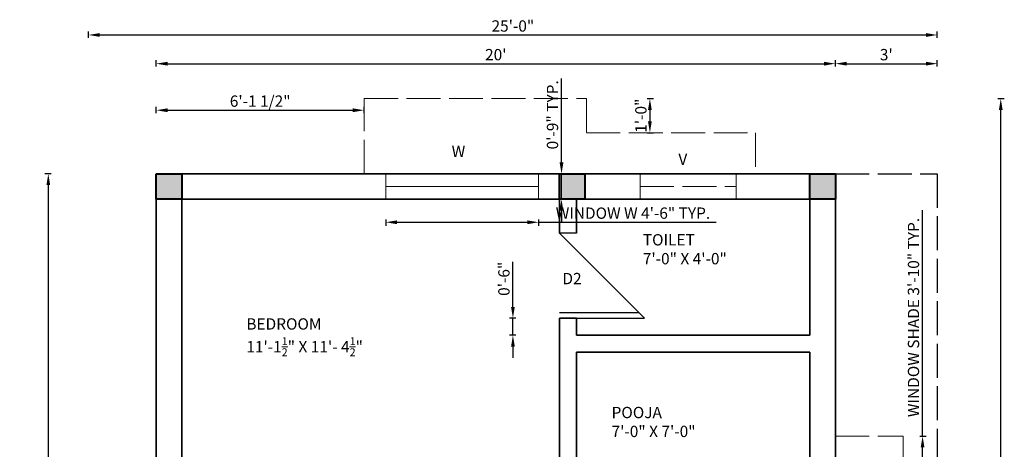
# Model space of a CAD drawing. Units: inches. Extents: x -52 to 299, y -380 to 67.
# Tile 2 of 2: x -49 to 299, y -84 to 67. Entities that reach past the tile are written whole.
import ezdxf

# ---------------------------------------------------------------- set-up
doc = ezdxf.new("R2010")
doc.units = ezdxf.units.IN
doc.linetypes.add('ACAD_ISO02W100', pattern=[15, 12, -3])
for name, color, linetype, lineweight in [('A-ANNO-DIMS', 2, 'Continuous', 18), ('A-ANNO-TEXT', 7, 'Continuous', 18), ('A-AREA-IDEN', 7, 'Continuous', 18), ('A-COLS', 7, 'Continuous', 40), ('A-DOOR', 3, 'Continuous', 25), ('A-GLAZ', 4, 'Continuous', 18), ('A-GLAZ-VENT', 4, 'ACAD_ISO02W100', 18), ('A-ROOF-OVHD', 8, 'ACAD_ISO02W100', 18), ('A-WALL', 7, 'Continuous', 35), ('C-PROP', 8, 'ACAD_ISO02W100', 25)]:
    doc.layers.add(name, color=color, linetype=linetype, lineweight=lineweight)
doc.styles.get("Standard").update_dxf_attribs({"font": 'arial.ttf'})
doc.dimstyles.new('ISO-25', dxfattribs={"dimtxt": 4, "dimasz": 4, "dimexe": 1.25, "dimexo": 0.625, "dimtad": 1, "dimlunit": 4, "dimtxsty": 'Standard', "dimcen": 2.5, "dimadec": 0, "dimazin": 0, "dimtfac": 1, "dimtmove": 0, "dimatfit": 3, "dimfxl": 1, "dimfxlon": 1, "dimarcsym": 0})

# ---------------------------------------------------------------- blocks, each defined once
blk = doc.blocks.new('*D1')
at = {"layer": 'A-ANNO-DIMS', "color": 0, "lineweight": -2, "transparency": 16777216}
for p, q in [((-0.38, 50.68), (-0.38, 52.93)), ((239.62, 50.68), (239.62, 52.93)), ((3.62, 51.68), (235.62, 51.68))]:
    blk.add_line(p, q, dxfattribs=at)
at = {"layer": 'A-ANNO-DIMS', "color": 0, "transparency": 16777216}
for points in [[(3.62, 52.35), (3.62, 51.01), (-0.38, 51.68)], [(235.62, 52.35), (235.62, 51.01), (239.62, 51.68)]]:
    blk.add_solid(points, dxfattribs=at)
at = {"layer": 'Defpoints', "color": 0, "transparency": 16777216}
for p in [(239.62, 51.68), (-0.38, 12.8), (239.62, 12.8)]:
    blk.add_point(p, dxfattribs=at)
at = {"layer": 'A-ANNO-DIMS', "color": 0, "transparency": 16777216, "insert": (119.62, 54.35), "char_height": 4, "attachment_point": 5}
blk.add_mtext("20'", dxfattribs=at)
blk = doc.blocks.new('*D2')
at = {"layer": 'A-ANNO-DIMS', "color": 0, "lineweight": -2, "transparency": 16777216}
for p, q in [((239.62, 50.68), (239.62, 52.93)), ((275.62, 50.68), (275.62, 52.93)), ((243.62, 51.68), (271.62, 51.68))]:
    blk.add_line(p, q, dxfattribs=at)
at = {"layer": 'A-ANNO-DIMS', "color": 0, "transparency": 16777216}
for points in [[(243.62, 52.35), (243.62, 51.01), (239.62, 51.68)], [(271.62, 52.35), (271.62, 51.01), (275.62, 51.68)]]:
    blk.add_solid(points, dxfattribs=at)
at = {"layer": 'Defpoints', "color": 0, "transparency": 16777216}
for p in [(275.62, 51.68), (239.62, 12.8), (275.62, 12.8)]:
    blk.add_point(p, dxfattribs=at)
at = {"layer": 'A-ANNO-DIMS', "color": 0, "transparency": 16777216, "insert": (257.62, 54.35), "char_height": 4, "attachment_point": 5}
blk.add_mtext("3'", dxfattribs=at)
blk = doc.blocks.new('*D3')
at = {"layer": 'A-ANNO-DIMS', "color": 0, "lineweight": -2, "transparency": 16777216}
for p, q in [((-37.52, 12.8), (-39.77, 12.8)), ((-38.52, 8.8), (-38.52, -278.7)), ((-37.52, -282.7), (-39.77, -282.7))]:
    blk.add_line(p, q, dxfattribs=at)
at = {"layer": 'A-ANNO-DIMS', "color": 0, "transparency": 16777216}
for points in [[(-39.19, 8.8), (-37.85, 8.8), (-38.52, 12.8)], [(-39.19, -278.7), (-37.85, -278.7), (-38.52, -282.7)]]:
    blk.add_solid(points, dxfattribs=at)
at = {"layer": 'Defpoints', "color": 0, "transparency": 16777216}
for p in [(-0.38, 12.8), (-38.52, -282.7), (-0.38, -282.7)]:
    blk.add_point(p, dxfattribs=at)
at = {"layer": 'A-ANNO-DIMS', "color": 0, "transparency": 16777216, "insert": (-43.83, -134.95), "char_height": 4, "attachment_point": 5, "rotation": 90}
blk.add_mtext('24\'-7{\\H1x;\\S1/2;}"', dxfattribs=at)
blk = doc.blocks.new('COL-9X9')
h = blk.add_hatch(color=256)
h.dxf.hatch_style = 1
h.paths.add_polyline_path([(0, 0), (9, 0), (9, 9), (0, 9)])
blk.add_lwpolyline([(0, 9), (9, 9), (9, 0), (0, 0)], close=True)
blk = doc.blocks.new('WIN-54')
blk.add_line((0, 4.5), (54, 4.5))
blk.add_lwpolyline([(0, 9), (54, 9), (54, 0), (0, 0)], close=True)
blk = doc.blocks.new('DOOR-D2-30')
for p, q in [((0, 0), (0, 30)), ((30, 0), (0, 30)), ((2, 0), (2, 28)), ((0, 6), (0, 0)), ((30, 6), (30, 0))]:
    blk.add_line(p, q)
blk = doc.blocks.new('WINDOW-SHADE-34')
blk.add_lwpolyline([(0, 45.87), (23.94, 45.87), (23.94, 0), (0, 0)], close=True)
blk = doc.blocks.new('*D12')
at = {"layer": 'A-ANNO-DIMS', "color": 0, "lineweight": -2, "transparency": 16777216}
for p, q in [((80.75, -3.3), (80.75, -5.55)), ((134.75, -3.3), (134.75, -5.55)), ((84.75, -4.3), (130.75, -4.3)), ((134.75, -4.3), (197.44, -4.3))]:
    blk.add_line(p, q, dxfattribs=at)
at = {"layer": 'A-ANNO-DIMS', "color": 0, "transparency": 16777216}
for points in [[(84.75, -3.63), (84.75, -4.97), (80.75, -4.3)], [(130.75, -3.63), (130.75, -4.97), (134.75, -4.3)]]:
    blk.add_solid(points, dxfattribs=at)
at = {"layer": 'Defpoints', "color": 0, "transparency": 16777216}
for p in [(80.75, 3.8), (134.75, 3.8), (134.75, -4.3)]:
    blk.add_point(p, dxfattribs=at)
at = {"layer": 'A-ANNO-DIMS', "color": 0, "transparency": 16777216, "insert": (168.09, -1.6), "char_height": 4, "attachment_point": 5}
blk.add_mtext('WINDOW W 4\'-6" TYP.', dxfattribs=at)
blk = doc.blocks.new('*D13')
at = {"layer": 'A-ANNO-DIMS', "color": 0, "lineweight": -2, "transparency": 16777216}
for p, q in [((142.85, 16.8), (142.85, 46.43)), ((141.85, 12.8), (144.1, 12.8)), ((142.85, 3.8), (142.85, 12.8)), ((141.85, 3.8), (144.1, 3.8)), ((142.85, -0.2), (142.85, -4.2))]:
    blk.add_line(p, q, dxfattribs=at)
at = {"layer": 'A-ANNO-DIMS', "color": 0, "transparency": 16777216}
for points in [[(142.18, 16.8), (143.51, 16.8), (142.85, 12.8)], [(142.18, -0.2), (143.51, -0.2), (142.85, 3.8)]]:
    blk.add_solid(points, dxfattribs=at)
at = {"layer": 'Defpoints', "color": 0, "transparency": 16777216}
for p in [(134.75, 12.8), (142.85, 12.8), (134.75, 3.8)]:
    blk.add_point(p, dxfattribs=at)
at = {"layer": 'A-ANNO-DIMS', "color": 0, "transparency": 16777216, "insert": (140.18, 33.62), "char_height": 4, "attachment_point": 5, "rotation": 90}
blk.add_mtext('0\'-9" TYP.', dxfattribs=at)
blk = doc.blocks.new('*D18')
at = {"layer": 'A-ANNO-DIMS', "color": 0, "lineweight": -2, "transparency": 16777216}
for p, q in [((270.45, -79.8), (270.45, -0.02)), ((269.45, -79.8), (271.7, -79.8)), ((270.45, -121.66), (270.45, -83.8)), ((269.45, -125.66), (271.7, -125.66))]:
    blk.add_line(p, q, dxfattribs=at)
at = {"layer": 'A-ANNO-DIMS', "color": 0, "transparency": 16777216}
for points in [[(269.78, -83.8), (271.11, -83.8), (270.45, -79.8)], [(269.78, -121.66), (271.11, -121.66), (270.45, -125.66)]]:
    blk.add_solid(points, dxfattribs=at)
at = {"layer": 'Defpoints', "color": 0, "transparency": 16777216}
for p in [(263.57, -79.8), (270.45, -79.8), (263.57, -125.66)]:
    blk.add_point(p, dxfattribs=at)
at = {"layer": 'A-ANNO-DIMS', "color": 0, "transparency": 16777216, "insert": (267.75, -37.91), "char_height": 4, "attachment_point": 5, "rotation": 90}
blk.add_mtext('WINDOW SHADE 3\'-10" TYP.', dxfattribs=at)
blk = doc.blocks.new('*D20')
at = {"layer": 'A-ANNO-DIMS', "color": 0, "lineweight": -2, "transparency": 16777216}
for p, q in [((-24.32, 60.81), (-24.32, 63.06)), ((275.62, 60.81), (275.62, 63.06)), ((-20.32, 61.81), (271.62, 61.81))]:
    blk.add_line(p, q, dxfattribs=at)
at = {"layer": 'A-ANNO-DIMS', "color": 0, "transparency": 16777216}
for points in [[(-20.32, 62.47), (-20.32, 61.14), (-24.32, 61.81)], [(271.62, 62.47), (271.62, 61.14), (275.62, 61.81)]]:
    blk.add_solid(points, dxfattribs=at)
at = {"layer": 'Defpoints', "color": 0, "transparency": 16777216}
for p in [(275.62, 61.81), (275.62, 12.8), (-24.32, -215.36)]:
    blk.add_point(p, dxfattribs=at)
at = {"layer": 'A-ANNO-DIMS', "color": 0, "transparency": 16777216, "insert": (125.65, 64.47), "char_height": 4, "attachment_point": 5}
blk.add_mtext('25\'-0"', dxfattribs=at)
blk = doc.blocks.new('*D21')
at = {"layer": 'A-ANNO-DIMS', "color": 0, "lineweight": -2, "transparency": 16777216}
for p, q in [((297.07, 39.36), (299.32, 39.36)), ((298.07, -350.7), (298.07, 35.36)), ((297.07, -354.7), (299.32, -354.7))]:
    blk.add_line(p, q, dxfattribs=at)
at = {"layer": 'A-ANNO-DIMS', "color": 0, "transparency": 16777216}
for points in [[(297.41, 35.36), (298.74, 35.36), (298.07, 39.36)], [(297.41, -350.7), (298.74, -350.7), (298.07, -354.7)]]:
    blk.add_solid(points, dxfattribs=at)
at = {"layer": 'Defpoints', "color": 0, "transparency": 16777216}
for p in [(151.63, 39.36), (298.07, 39.36), (275.62, -354.7)]:
    blk.add_point(p, dxfattribs=at)
at = {"layer": 'A-ANNO-DIMS', "color": 0, "transparency": 16777216, "insert": (295.4, -157.67), "char_height": 4, "attachment_point": 5, "rotation": 90}
blk.add_mtext('32\'-10"', dxfattribs=at)
blk = doc.blocks.new('*D24')
at = {"layer": 'A-ANNO-DIMS', "color": 0, "lineweight": -2, "transparency": 16777216}
for p, q in [((8.62, -376.15), (8.62, -378.4)), ((12.62, -377.15), (76.75, -377.15)), ((80.75, -376.15), (80.75, -378.4))]:
    blk.add_line(p, q, dxfattribs=at)
at = {"layer": 'A-ANNO-DIMS', "color": 0, "transparency": 16777216}
for points in [[(12.62, -376.48), (12.62, -377.82), (8.62, -377.15)], [(76.75, -376.48), (76.75, -377.82), (80.75, -377.15)]]:
    blk.add_solid(points, dxfattribs=at)
at = {"layer": 'Defpoints', "color": 0, "transparency": 16777216}
for p in [(8.62, 3.8), (80.75, 3.8), (80.75, -377.15)]:
    blk.add_point(p, dxfattribs=at)
at = {"layer": 'A-ANNO-DIMS', "color": 0, "transparency": 16777216, "insert": (44.69, -374.48), "char_height": 4, "attachment_point": 5}
blk.add_mtext('6\'-0"', dxfattribs=at)
blk = doc.blocks.new('*D25')
at = {"layer": 'A-ANNO-DIMS', "color": 0, "lineweight": -2, "transparency": 16777216}
for p, q in [((170.58, -376.15), (170.58, -378.4)), ((174.58, -377.15), (200.58, -377.15)), ((204.58, -376.15), (204.58, -378.4))]:
    blk.add_line(p, q, dxfattribs=at)
at = {"layer": 'A-ANNO-DIMS', "color": 0, "transparency": 16777216}
for points in [[(174.58, -376.48), (174.58, -377.82), (170.58, -377.15)], [(200.58, -376.48), (200.58, -377.82), (204.58, -377.15)]]:
    blk.add_solid(points, dxfattribs=at)
at = {"layer": 'Defpoints', "color": 0, "transparency": 16777216}
for p in [(170.58, 3.8), (204.58, 3.8), (204.58, -377.15)]:
    blk.add_point(p, dxfattribs=at)
at = {"layer": 'A-ANNO-DIMS', "color": 0, "transparency": 16777216, "insert": (187.58, -374.48), "char_height": 4, "attachment_point": 5}
blk.add_mtext('2\'-10"', dxfattribs=at)
blk = doc.blocks.new('*D26')
at = {"layer": 'A-ANNO-DIMS', "color": 0, "lineweight": -2, "transparency": 16777216}
for p, q in [((204.58, -376.15), (204.58, -378.4)), ((208.58, -377.15), (226.62, -377.15)), ((230.62, -376.15), (230.62, -378.4))]:
    blk.add_line(p, q, dxfattribs=at)
at = {"layer": 'A-ANNO-DIMS', "color": 0, "transparency": 16777216}
for points in [[(208.58, -376.48), (208.58, -377.82), (204.58, -377.15)], [(226.62, -376.48), (226.62, -377.82), (230.62, -377.15)]]:
    blk.add_solid(points, dxfattribs=at)
at = {"layer": 'Defpoints', "color": 0, "transparency": 16777216}
for p in [(204.58, 3.8), (230.62, 3.8), (230.62, -377.15)]:
    blk.add_point(p, dxfattribs=at)
at = {"layer": 'A-ANNO-DIMS', "color": 0, "transparency": 16777216, "insert": (217.6, -374.52), "char_height": 4, "attachment_point": 5}
blk.add_mtext('2\'-2"', dxfattribs=at)
blk = doc.blocks.new('*D36')
at = {"layer": 'A-ANNO-DIMS', "color": 0, "lineweight": -2, "transparency": 16777216}
for p, q in [((125.67, -34.2), (125.67, -18.32)), ((126.67, -38.2), (124.42, -38.2)), ((125.67, -44.2), (125.67, -38.2)), ((126.67, -44.2), (124.42, -44.2)), ((125.67, -48.2), (125.67, -52.2))]:
    blk.add_line(p, q, dxfattribs=at)
at = {"layer": 'A-ANNO-DIMS', "color": 0, "transparency": 16777216}
for points in [[(125.01, -34.2), (126.34, -34.2), (125.67, -38.2)], [(125.01, -48.2), (126.34, -48.2), (125.67, -44.2)]]:
    blk.add_solid(points, dxfattribs=at)
at = {"layer": 'Defpoints', "color": 0, "transparency": 16777216}
for p in [(125.67, -38.2), (148.12, -38.2), (148.12, -44.2)]:
    blk.add_point(p, dxfattribs=at)
at = {"layer": 'A-ANNO-DIMS', "color": 0, "transparency": 16777216, "insert": (123.01, -24.26), "char_height": 4, "attachment_point": 5, "rotation": 90}
blk.add_mtext('0\'-6"', dxfattribs=at)
blk = doc.blocks.new('*D40')
at = {"layer": 'A-ANNO-DIMS', "color": 0, "lineweight": -2, "transparency": 16777216}
for p, q in [((173.08, 39.36), (175.33, 39.36)), ((174.08, 35.36), (174.08, 31.28)), ((173.08, 27.28), (175.33, 27.28))]:
    blk.add_line(p, q, dxfattribs=at)
at = {"layer": 'A-ANNO-DIMS', "color": 0, "transparency": 16777216}
for points in [[(173.41, 35.36), (174.74, 35.36), (174.08, 39.36)], [(173.41, 31.28), (174.74, 31.28), (174.08, 27.28)]]:
    blk.add_solid(points, dxfattribs=at)
at = {"layer": 'Defpoints', "color": 0, "transparency": 16777216}
for p in [(151.63, 39.36), (151.63, 27.28), (174.08, 27.28)]:
    blk.add_point(p, dxfattribs=at)
at = {"layer": 'A-ANNO-DIMS', "color": 0, "transparency": 16777216, "insert": (171.41, 33.32), "char_height": 4, "attachment_point": 5, "rotation": 90}
blk.add_mtext('1\'-0"', dxfattribs=at)
blk = doc.blocks.new('*D41')
at = {"layer": 'A-ANNO-DIMS', "color": 0, "lineweight": -2, "transparency": 16777216}
for p, q in [((-0.38, 34.25), (-0.38, 36.5)), ((3.62, 35.25), (69.09, 35.25)), ((73.09, 34.25), (73.09, 36.5))]:
    blk.add_line(p, q, dxfattribs=at)
at = {"layer": 'A-ANNO-DIMS', "color": 0, "transparency": 16777216}
for points in [[(3.62, 35.92), (3.62, 34.58), (-0.38, 35.25)], [(69.09, 35.92), (69.09, 34.58), (73.09, 35.25)]]:
    blk.add_solid(points, dxfattribs=at)
at = {"layer": 'Defpoints', "color": 0, "transparency": 16777216}
for p in [(73.09, 35.25), (-0.38, 12.8), (73.09, 12.8)]:
    blk.add_point(p, dxfattribs=at)
at = {"layer": 'A-ANNO-DIMS', "color": 0, "transparency": 16777216, "insert": (36.36, 37.94), "char_height": 4, "attachment_point": 5}
blk.add_mtext('6\'-1 1/2"', dxfattribs=at)
blk = doc.blocks.new('*D42')
at = {"layer": 'A-ANNO-DIMS', "color": 0, "lineweight": -2, "transparency": 16777216}
for p, q in [((73.09, -376.15), (73.09, -378.4)), ((77.09, -377.15), (147.63, -377.15)), ((151.63, -376.15), (151.63, -378.4))]:
    blk.add_line(p, q, dxfattribs=at)
at = {"layer": 'A-ANNO-DIMS', "color": 0, "transparency": 16777216}
for points in [[(77.09, -376.48), (77.09, -377.82), (73.09, -377.15)], [(147.63, -376.48), (147.63, -377.82), (151.63, -377.15)]]:
    blk.add_solid(points, dxfattribs=at)
at = {"layer": 'Defpoints', "color": 0, "transparency": 16777216}
for p in [(73.09, 39.36), (151.63, 39.36), (151.63, -377.15)]:
    blk.add_point(p, dxfattribs=at)
at = {"layer": 'A-ANNO-DIMS', "color": 0, "transparency": 16777216, "insert": (112.36, -374.46), "char_height": 4, "attachment_point": 5}
blk.add_mtext('6\'-6 1/2"', dxfattribs=at)
blk = doc.blocks.new('*D43')
at = {"layer": 'A-ANNO-DIMS', "color": 0, "lineweight": -2, "transparency": 16777216}
for p, q in [((151.63, -376.15), (151.63, -378.4)), ((155.63, -377.15), (207.36, -377.15)), ((211.36, -376.15), (211.36, -378.4))]:
    blk.add_line(p, q, dxfattribs=at)
at = {"layer": 'A-ANNO-DIMS', "color": 0, "transparency": 16777216}
for points in [[(155.63, -376.48), (155.63, -377.82), (151.63, -377.15)], [(207.36, -376.48), (207.36, -377.82), (211.36, -377.15)]]:
    blk.add_solid(points, dxfattribs=at)
at = {"layer": 'Defpoints', "color": 0, "transparency": 16777216}
for p in [(151.63, 27.28), (211.36, 27.28), (211.36, -377.15)]:
    blk.add_point(p, dxfattribs=at)
at = {"layer": 'A-ANNO-DIMS', "color": 0, "transparency": 16777216, "insert": (181.49, -374.46), "char_height": 4, "attachment_point": 5}
blk.add_mtext('4\'-11 1/2"', dxfattribs=at)

msp = doc.modelspace()

# ---------------------------------------------------------------- linework, layer by layer
at = {"layer": 'A-GLAZ'}
msp.add_lwpolyline([(170.585, 12.801), (204.585, 12.801), (204.585, 3.801), (170.585, 3.801)], close=True, dxfattribs=at)
at = {"layer": 'A-GLAZ-VENT'}
msp.add_line((170.585, 8.301), (204.585, 8.301), dxfattribs=at)
at = {"layer": 'A-ROOF-OVHD'}
for p, q in [((73.092, 12.801), (73.092, 39.357)), ((73.092, 39.357), (151.625, 39.357)), ((151.625, 39.357), (151.625, 27.284)), ((151.625, 27.284), (211.364, 27.284)), ((211.364, 27.284), (211.364, 12.801))]:
    msp.add_line(p, q, dxfattribs=at)
at = {"layer": 'A-WALL'}
for p, q in [((-0.377, 12.801), (239.623, 12.801)), ((-0.377, -282.699), (-0.377, 12.801)), ((239.623, 12.801), (239.623, -282.699)), ((8.623, 3.801), (142.123, 3.801)), ((8.623, -273.699), (8.623, 3.801)), ((142.123, 3.801), (148.123, 3.801)), ((142.123, -8.199), (142.123, 3.801)), ((148.123, 3.801), (230.623, 3.801)), ((148.123, -8.199), (148.123, 3.801)), ((230.623, 3.801), (230.623, -44.199)), ((142.123, -138.699), (142.123, -38.199)), ((148.123, -44.199), (148.123, -38.199)), ((148.123, -44.199), (230.623, -44.199)), ((148.123, -138.699), (148.123, -50.199)), ((148.123, -50.199), (230.623, -50.199)), ((230.623, -50.199), (230.623, -273.699))]:
    msp.add_line(p, q, dxfattribs=at)
at = {"layer": 'C-PROP'}
for p, q in [((239.623, 12.801), (275.623, 12.801)), ((275.623, 12.801), (275.623, -354.699))]:
    msp.add_line(p, q, dxfattribs=at)

# ---------------------------------------------------------------- block references
at = {"layer": 'A-COLS'}
for p in [(-0.377, 3.801), (142.093, 3.801), (230.623, 3.801)]:
    msp.add_blockref('COL-9X9', p, dxfattribs=at)
at = {"layer": 'A-DOOR', "extrusion": (0, 0, -1), "zscale": -1, "rotation": 89.99999999999989}
msp.add_blockref('DOOR-D2-30', (-142.123, -38.199), dxfattribs=at)
at = {"layer": 'A-GLAZ'}
msp.add_blockref('WIN-54', (80.748, 3.801), dxfattribs=at)
at = {"layer": 'A-ROOF-OVHD'}
msp.add_blockref('WINDOW-SHADE-34', (239.623, -125.661), dxfattribs=at)

# ---------------------------------------------------------------- texts
at = {"layer": 'A-ANNO-TEXT', "char_height": 4, "attachment_point": 1}
for s, width, insert in [('W', 15.80542, (104.03, 22.704)), ('V', 9.29189, (184.149, 19.959)), ('D2', 7.3032, (143.167, -22.176))]:
    msp.add_mtext_dynamic_manual_height_columns(s, width=width, gutter_width=12.5, heights=[0], dxfattribs=dict(at, insert=insert))
at = {"layer": 'A-AREA-IDEN', "char_height": 4, "attachment_point": 1}
for s, width, insert in [('TOILET\\P7\'-0" X 4\'-0"', 42.70641, (171.585, -8.482)), ('\\A1;BEDROOM\\P11\'-1{\\H0.7x;\\S1/2;}" X 11\'- 4{\\H0.7x;\\S1/2;}"', 60.67252, (31.466, -38.199)), ('POOJA\\P7\'-0" X 7\'-0"', 49.77219, (160.533, -69.457))]:
    msp.add_mtext_dynamic_manual_height_columns(s, width=width, gutter_width=12.5, heights=[0], dxfattribs=dict(at, insert=insert))

# ---------------------------------------------------------------- dimensions: what is measured, and where the dimension line sits
at = {"layer": 'A-ANNO-DIMS'}
for base, p1, p2, override, picture, middle in [((275.623, 61.807), (-24.321, -215.357), (275.623, 12.801), {"dimdec": 1, "dimlfac": 1, "dimrnd": 0, "dimzin": 1, "dimdsep": 46, "dimlunit": 4, "dimfrac": 2}, '*D20', (125.651, 64.474)), ((239.623, 51.68), (-0.377, 12.801), (239.623, 12.801), {"dimclrd": 0, "dimclre": 0, "dimclrt": 0}, '*D1', (119.623, 54.348)), ((275.623, 51.68), (239.623, 12.801), (275.623, 12.801), {"dimclrd": 0, "dimclre": 0, "dimclrt": 0}, '*D2', (257.623, 54.349)), ((151.625, -377.149), (73.092, 39.357), (151.625, 39.357), {"dimdec": 1, "dimlfac": 1, "dimrnd": 0, "dimzin": 1, "dimdsep": 46, "dimlunit": 4, "dimfrac": 2}, '*D42', (112.359, -374.456)), ((211.364, -377.149), (151.625, 27.284), (211.364, 27.284), {"dimdec": 1, "dimlfac": 1, "dimrnd": 0, "dimzin": 1, "dimdsep": 46, "dimlunit": 4, "dimfrac": 2}, '*D43', (181.495, -374.456)), ((80.748, -377.149), (8.623, 3.801), (80.748, 3.801), {"dimdec": 1, "dimlfac": 1, "dimrnd": 0, "dimzin": 1, "dimdsep": 46, "dimlunit": 4, "dimfrac": 2}, '*D24', (44.686, -374.482)), ((204.585, -377.149), (170.585, 3.801), (204.585, 3.801), {"dimdec": 1, "dimlfac": 1, "dimrnd": 0, "dimzin": 1, "dimdsep": 46, "dimlunit": 4, "dimfrac": 2}, '*D25', (187.585, -374.482)), ((230.623, -377.149), (204.585, 3.801), (230.623, 3.801), {"dimdec": 1, "dimlfac": 1, "dimrnd": 0, "dimzin": 1, "dimdsep": 46, "dimlunit": 4, "dimfrac": 2}, '*D26', (217.604, -374.516))]:
    dim = msp.add_linear_dim(base=base, p1=p1, p2=p2, dimstyle='ISO-25', override=override, dxfattribs=at)
    dim.commit()
    dim.dimension.update_dxf_attribs({"geometry": picture, "text_midpoint": middle})
for base, p1, p2, text, picture, middle in [((142.848, 12.801), (134.748, 3.801), (134.748, 12.801), '<> TYP.', '*D13', (140.181, 33.617)), ((270.447, -79.796), (263.567, -125.661), (263.567, -79.796), 'WINDOW SHADE <> TYP.', '*D18', (267.751, -37.906))]:
    dim = msp.add_linear_dim(base=base, p1=p1, p2=p2, angle=90, text=text, dimstyle='ISO-25', override={"dimdec": 1, "dimlfac": 1, "dimrnd": 0, "dimzin": 1, "dimdsep": 46, "dimlunit": 4, "dimfrac": 2}, dxfattribs=at)
    dim.commit()
    dim.dimension.update_dxf_attribs({"geometry": picture, "text_midpoint": middle})
for base, p1, p2, angle, override, picture, middle in [((73.092, 35.251), (-0.377, 12.801), (73.092, 12.801), 0, {"dimdec": 1, "dimlfac": 1, "dimrnd": 0, "dimzin": 1, "dimdsep": 46, "dimlunit": 4, "dimfrac": 2}, '*D41', (36.358, 37.944)), ((298.073, 39.357), (275.623, -354.699), (151.625, 39.357), 90, {"dimdec": 1, "dimlfac": 1, "dimrnd": 0, "dimzin": 1, "dimdsep": 46, "dimlunit": 4, "dimfrac": 2}, '*D21', (295.404, -157.671)), ((174.075, 27.284), (151.625, 39.357), (151.625, 27.284), 270, {"dimdec": 1, "dimlfac": 1, "dimrnd": 0, "dimzin": 1, "dimdsep": 46, "dimlunit": 4, "dimfrac": 2}, '*D40', (171.408, 33.32)), ((-38.52, -282.699), (-0.377, 12.801), (-0.38, -282.699), 90, {"dimclrd": 0, "dimclre": 0, "dimclrt": 0}, '*D3', (-43.828, -134.949)), ((125.673, -38.199), (148.123, -44.199), (148.123, -38.199), 90, {"dimdec": 1, "dimlfac": 1, "dimrnd": 0, "dimzin": 1, "dimdsep": 46, "dimlunit": 4, "dimfrac": 2}, '*D36', (123.006, -24.258))]:
    dim = msp.add_linear_dim(base=base, p1=p1, p2=p2, angle=angle, dimstyle='ISO-25', override=override, dxfattribs=at)
    dim.commit()
    dim.dimension.update_dxf_attribs({"geometry": picture, "text_midpoint": middle})
dim = msp.add_linear_dim(base=(134.748, -4.299), p1=(80.748, 3.801), p2=(134.748, 3.801), text='WINDOW W <> TYP.', dimstyle='ISO-25', override={"dimdec": 1, "dimlfac": 1, "dimrnd": 0, "dimzin": 1, "dimdsep": 46, "dimlunit": 4, "dimfrac": 2}, dxfattribs=at)
dim.commit()
dim.dimension.update_dxf_attribs({"geometry": '*D12', "text_midpoint": (168.095, -1.605)})

doc.saveas('drawing.dxf')
